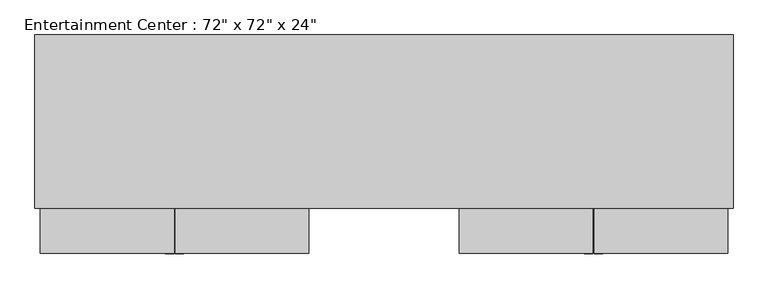
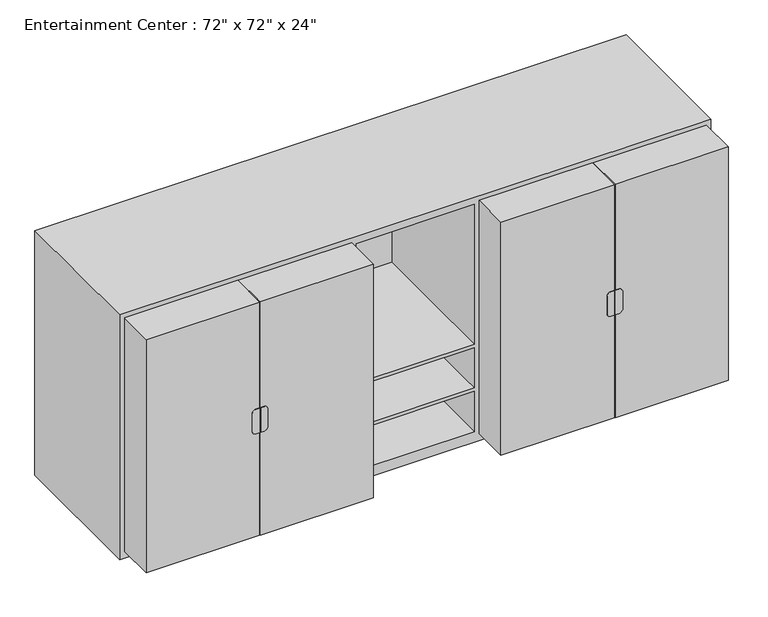
"""IFC4 building model written with IfcOpenShell, lengths in millimetres: furniture geometry."""

from ifc_helpers import new_model, si_unit, point, frame, frame_2d, origin, place, context, project, spatial, polyline, circle_curve, trimmed, segment, composite_curve, outline, extrude, faceted_brep, source, transform, mapped, element, save


def furniture_eacb8e26(model_context):
    return source(origin(), model_context, "Body", "SolidModel", [
        extrude(outline(polyline([(-2000.25, -781.05), (-1222.375, -781.05), (-1222.375, -1041.4), (-2000.25, -1041.4), (-2000.25, -781.05)])), frame((0.0, 0.0, 50.8), z_axis=(0.0, 0.0, 1.0), x_axis=(1.0, 0.0, 0.0)), (0.0, 0.0, 1.0), 1695.45),
        extrude(outline(polyline([(-1216.025, -781.05), (-438.15, -781.05), (-438.15, -1041.4), (-1216.025, -1041.4), (-1216.025, -781.05)])), frame((0.0, 0.0, 50.8), z_axis=(0.0, 0.0, 1.0), x_axis=(1.0, 0.0, 0.0)), (0.0, 0.0, 1.0), 1695.45),
        extrude(outline(polyline([(1222.375, -781.05), (2000.25, -781.05), (2000.25, -1041.4), (1222.375, -1041.4), (1222.375, -781.05)])), frame((0.0, 0.0, 50.8), z_axis=(0.0, 0.0, 1.0), x_axis=(1.0, 0.0, 0.0)), (0.0, 0.0, 1.0), 1695.45),
        extrude(outline(polyline([(438.15, -781.05), (1216.025, -781.05), (1216.025, -1041.4), (438.15, -1041.4), (438.15, -781.05)])), frame((0.0, 0.0, 50.8), z_axis=(0.0, 0.0, 1.0), x_axis=(1.0, 0.0, 0.0)), (0.0, 0.0, 1.0), 1695.45),
        extrude(outline(composite_curve([segment(polyline([(977.9, -1191.7986452), (977.9, -1216.025), (800.1, -1216.025), (800.1, -1191.7986452)]), True, "CONTINUOUS"), segment(trimmed(circle_curve(frame_2d((825.5, -1191.7986452)), 25.4), [point((800.1, -1191.7986452))], [point((825.5, -1166.3986452))], False, "CARTESIAN"), True, "CONTINUOUS"), segment(polyline([(825.5, -1166.3986452), (952.5, -1166.3986452)]), True, "CONTINUOUS"), segment(trimmed(circle_curve(frame_2d((952.5, -1191.7986452)), 25.4), [point((952.5, -1166.3986452))], [point((977.9, -1191.7986452))], False, "CARTESIAN"), True, "CONTINUOUS")], self_intersect=False)), frame((0.0, -1044.575, 0.0), z_axis=(0.0, 1.0, 0.0), x_axis=(0.0, 0.0, 1.0)), (0.0, 0.0, 1.0), 3.175),
        extrude(outline(composite_curve([segment(trimmed(circle_curve(frame_2d((952.5, -1246.98125)), 25.4), [point((977.9, -1246.98125))], [point((952.5, -1272.38125))], False, "CARTESIAN"), True, "CONTINUOUS"), segment(polyline([(952.5, -1272.38125), (825.5, -1272.38125)]), True, "CONTINUOUS"), segment(trimmed(circle_curve(frame_2d((825.5, -1246.98125)), 25.4), [point((825.5, -1272.38125))], [point((800.1, -1246.98125))], False, "CARTESIAN"), True, "CONTINUOUS"), segment(polyline([(800.1, -1246.98125), (800.1, -1222.375), (977.9, -1222.375), (977.9, -1246.98125)]), True, "CONTINUOUS")], self_intersect=False)), frame((0.0, -1044.575, 0.0), z_axis=(0.0, 1.0, 0.0), x_axis=(0.0, 0.0, 1.0)), (0.0, 0.0, 1.0), 3.175),
        extrude(outline(composite_curve([segment(trimmed(circle_curve(frame_2d((952.5, 1191.7986452)), 25.4), [point((977.9, 1191.7986452))], [point((952.5, 1166.3986452))], False, "CARTESIAN"), True, "CONTINUOUS"), segment(polyline([(952.5, 1166.3986452), (825.5, 1166.3986452)]), True, "CONTINUOUS"), segment(trimmed(circle_curve(frame_2d((825.5, 1191.7986452)), 25.4), [point((825.5, 1166.3986452))], [point((800.1, 1191.7986452))], False, "CARTESIAN"), True, "CONTINUOUS"), segment(polyline([(800.1, 1191.7986452), (800.1, 1216.025), (977.9, 1216.025), (977.9, 1191.7986452)]), True, "CONTINUOUS")], self_intersect=False)), frame((0.0, -1044.575, 0.0), z_axis=(0.0, 1.0, 0.0), x_axis=(0.0, 0.0, 1.0)), (0.0, 0.0, 1.0), 3.175),
        extrude(outline(composite_curve([segment(polyline([(977.9, 1246.98125), (977.9, 1222.375), (800.1, 1222.375), (800.1, 1246.98125)]), True, "CONTINUOUS"), segment(trimmed(circle_curve(frame_2d((825.5, 1246.98125)), 25.4), [point((800.1, 1246.98125))], [point((825.5, 1272.38125))], False, "CARTESIAN"), True, "CONTINUOUS"), segment(polyline([(825.5, 1272.38125), (952.5, 1272.38125)]), True, "CONTINUOUS"), segment(trimmed(circle_curve(frame_2d((952.5, 1246.98125)), 25.4), [point((952.5, 1272.38125))], [point((977.9, 1246.98125))], False, "CARTESIAN"), True, "CONTINUOUS")], self_intersect=False)), frame((0.0, -1044.575, 0.0), z_axis=(0.0, 1.0, 0.0), x_axis=(0.0, 0.0, 1.0)), (0.0, 0.0, 1.0), 3.175),
        faceted_brep([(2032.0, -781.05, 0.0), (2032.0, -781.05, 1778.0), (-2032.0, -781.05, 1778.0), (-2032.0, -781.05, 0.0), (-457.2, -781.05, 1727.2), (-457.2, -781.05, 1346.2), (-1981.2, -781.05, 1346.2), (-1981.2, -781.05, 1727.2), (-457.2, -781.05, 76.2), (-1981.2, -781.05, 76.2), (-1981.2, -781.05, 431.8), (-457.2, -781.05, 431.8), (1981.2, -781.05, 1346.2), (457.2, -781.05, 1346.2), (457.2, -781.05, 1727.2), (1981.2, -781.05, 1727.2), (-406.4, -781.05, 711.2), (-406.4, -781.05, 1727.2), (406.4, -781.05, 1727.2), (406.4, -781.05, 711.2), (406.4, -781.05, 76.2), (-406.4, -781.05, 76.2), (-406.4, -781.05, 368.3), (406.4, -781.05, 368.3), (1981.2, -781.05, 76.2), (457.2, -781.05, 76.2), (457.2, -781.05, 431.8), (1981.2, -781.05, 431.8), (-1981.2, -781.05, 457.2), (-1981.2, -781.05, 876.3), (-457.2, -781.05, 876.3), (-457.2, -781.05, 457.2), (-457.2, -781.05, 1320.8), (-457.2, -781.05, 901.7), (-1981.2, -781.05, 901.7), (-1981.2, -781.05, 1320.8), (457.2, -781.05, 1320.8), (1981.2, -781.05, 1320.8), (1981.2, -781.05, 901.7), (457.2, -781.05, 901.7), (457.2, -781.05, 876.3), (1981.2, -781.05, 876.3), (1981.2, -781.05, 457.2), (457.2, -781.05, 457.2), (406.4, -781.05, 393.7), (-406.4, -781.05, 393.7), (-406.4, -781.05, 685.8), (406.4, -781.05, 685.8), (2032.0, 228.6, 0.0), (-2032.0, 228.6, 0.0), (-2032.0, 228.6, 1778.0), (2032.0, 228.6, 1778.0), (-457.2, 203.2, 1727.2), (-457.2, 203.2, 1346.2), (-1981.2, 203.2, 1346.2), (-1981.2, 203.2, 1727.2), (-457.2, 203.2, 76.2), (-1981.2, 203.2, 76.2), (-1981.2, 203.2, 431.8), (-457.2, 203.2, 431.8), (1981.2, 203.2, 1346.2), (457.2, 203.2, 1346.2), (457.2, 203.2, 1727.2), (1981.2, 203.2, 1727.2), (-406.4, 203.2, 711.2), (-406.4, 203.2, 1727.2), (406.4, 203.2, 1727.2), (406.4, 203.2, 711.2), (406.4, 203.2, 76.2), (-406.4, 203.2, 76.2), (-406.4, 203.2, 368.3), (406.4, 203.2, 368.3), (1981.2, 203.2, 76.2), (457.2, 203.2, 76.2), (457.2, 203.2, 431.8), (1981.2, 203.2, 431.8), (-1981.2, 203.2, 457.2), (-1981.2, 203.2, 876.3), (-457.2, 203.2, 876.3), (-457.2, 203.2, 457.2), (-457.2, 203.2, 1320.8), (-457.2, 203.2, 901.7), (-1981.2, 203.2, 901.7), (-1981.2, 203.2, 1320.8), (457.2, 203.2, 1320.8), (1981.2, 203.2, 1320.8), (1981.2, 203.2, 901.7), (457.2, 203.2, 901.7), (457.2, 203.2, 876.3), (1981.2, 203.2, 876.3), (1981.2, 203.2, 457.2), (457.2, 203.2, 457.2), (406.4, 203.2, 393.7), (-406.4, 203.2, 393.7), (-406.4, 203.2, 685.8), (406.4, 203.2, 685.8)], [[[0, 1, 2, 3], [4, 5, 6, 7], [8, 9, 10, 11], [12, 13, 14, 15], [16, 17, 18, 19], [20, 21, 22, 23], [24, 25, 26, 27], [28, 29, 30, 31], [32, 33, 34, 35], [36, 37, 38, 39], [40, 41, 42, 43], [44, 45, 46, 47]], [[48, 49, 50, 51]], [[1, 0, 48, 51]], [[2, 1, 51, 50]], [[3, 2, 50, 49]], [[0, 3, 49, 48]], [[5, 4, 52, 53]], [[6, 5, 53, 54]], [[7, 6, 54, 55]], [[4, 7, 55, 52]], [[9, 8, 56, 57]], [[10, 9, 57, 58]], [[11, 10, 58, 59]], [[8, 11, 59, 56]], [[13, 12, 60, 61]], [[14, 13, 61, 62]], [[15, 14, 62, 63]], [[12, 15, 63, 60]], [[17, 16, 64, 65]], [[18, 17, 65, 66]], [[19, 18, 66, 67]], [[16, 19, 67, 64]], [[21, 20, 68, 69]], [[22, 21, 69, 70]], [[23, 22, 70, 71]], [[20, 23, 71, 68]], [[25, 24, 72, 73]], [[26, 25, 73, 74]], [[27, 26, 74, 75]], [[24, 27, 75, 72]], [[29, 28, 76, 77]], [[30, 29, 77, 78]], [[31, 30, 78, 79]], [[28, 31, 79, 76]], [[33, 32, 80, 81]], [[34, 33, 81, 82]], [[35, 34, 82, 83]], [[32, 35, 83, 80]], [[37, 36, 84, 85]], [[38, 37, 85, 86]], [[39, 38, 86, 87]], [[36, 39, 87, 84]], [[41, 40, 88, 89]], [[42, 41, 89, 90]], [[43, 42, 90, 91]], [[40, 43, 91, 88]], [[45, 44, 92, 93]], [[46, 45, 93, 94]], [[47, 46, 94, 95]], [[44, 47, 95, 92]], [[53, 52, 55, 54]], [[57, 56, 59, 58]], [[61, 60, 63, 62]], [[65, 64, 67, 66]], [[69, 68, 71, 70]], [[73, 72, 75, 74]], [[77, 76, 79, 78]], [[81, 80, 83, 82]], [[85, 84, 87, 86]], [[89, 88, 91, 90]], [[93, 92, 95, 94]]]),
    ])


if __name__ == "__main__":
    model = new_model("IFC4")
    model_context = context("Model", 3, world=origin())
    ifc_project = project(units=[si_unit("LENGTHUNIT", "METRE", prefix="MILLI")], contexts=[model_context])
    site = spatial("IfcSite", under=ifc_project)
    building = spatial("IfcBuilding", under=site)
    placement = place(None, origin())
    furniture_shape = furniture_eacb8e26(model_context)
    element("IfcFurniture", 1, ObjectType="Entertainment Center : 72\" x 72\" x 24\"", at=placement, inside=building, context=model_context, shape_type="MappedRepresentation", body=[
        mapped(furniture_shape, transform((0.0, 0.0, 0.0), x_axis=(1.0, 0.0, 0.0), y_axis=(0.0, 1.0, 0.0), z_axis=(0.0, 0.0, 1.0))),
    ])
    save(model, "model.ifc")

# Revit data of these elements
# Type "Entertainment Center : 72\" x 72\" x 24\""
#   Assembly Code = "E2020200"
#   Center Width = 2' - 8"
#   Depth = 4' - 2"
#   Height = 5' - 10"
#   Width = 13' - 4"
#   Material = none
#   Default Elevation = 0
# Element 1 (IfcFurniture, "Entertainment Center : 72\" x 72\" x 24\"")
#   Materials on its faces: "Steel, Chrome Plated", "Glass - Clear, Grey"
# Materials
#   "Steel, Chrome Plated": class "Metal", colour RGB 216 216 216, transparency 0, Description = "Chromiuim plated steel", Cost = 0
#   "Glass - Clear, Grey": class "Glass", colour RGB 252 255 255, transparency 0.64
